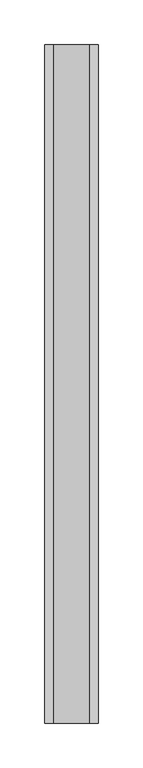
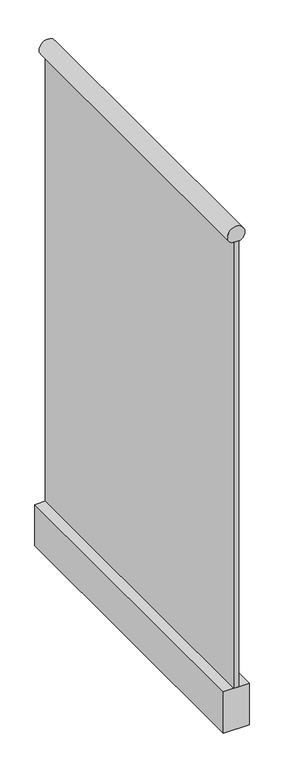
"""IFC4 building model written with IfcOpenShell, lengths in millimetres: railing geometry."""

from ifc_helpers import new_model, si_unit, point, frame, frame_2d, origin, place, context, project, spatial, polyline, circle_curve, trimmed, segment, composite_curve, outline, extrude, source, transform, mapped, element, save


def railing_f1bd4664(model_context):
    return source(origin(), model_context, "Body", "SweptSolid", [
        extrude(outline(composite_curve([segment(trimmed(circle_curve(frame_2d((5015.3205081, -1533.8712297)), 20.0), [point((4998.0, -1523.8712297))], [point((4998.0, -1543.8712297))], False, "CARTESIAN"), True, "CONTINUOUS"), segment(polyline([(4998.0, -1543.8712297), (4998.0, -1523.8712297)]), True, "CONTINUOUS")], self_intersect=False)), frame((0.0, -6422.0014262, 0.0), z_axis=(0.0, 1.0, 0.0), x_axis=(0.0, 0.0, 1.0)), (0.0, 0.0, 1.0), 760.0),
        extrude(outline(polyline([(-1527.8712297, -6422.0014262), (-1539.8712297, -6422.0014262), (-1539.8712297, -5662.0014262), (-1527.8712297, -5662.0014262), (-1527.8712297, -6422.0014262)])), frame((0.0, 0.0, 3900.0), z_axis=(0.0, 0.0, 1.0), x_axis=(1.0, 0.0, 0.0)), (0.0, 0.0, 1.0), 1098.0),
        extrude(outline(polyline([(-1503.8712297, -6422.0014262), (-1563.8712297, -6422.0014262), (-1563.8712297, -5662.0014262), (-1503.8712297, -5662.0014262), (-1503.8712297, -6422.0014262)])), frame((0.0, 0.0, 3798.0), z_axis=(0.0, 0.0, 1.0), x_axis=(1.0, 0.0, 0.0)), (0.0, 0.0, 1.0), 102.0),
    ])


if __name__ == "__main__":
    model = new_model("IFC4")
    model_context = context("Model", 3, world=origin())
    ifc_project = project(units=[si_unit("LENGTHUNIT", "METRE", prefix="MILLI")], contexts=[model_context])
    site = spatial("IfcSite", under=ifc_project)
    building = spatial("IfcBuilding", under=site)
    placement = place(None, origin())
    railing_shape = railing_f1bd4664(model_context)
    element("IfcRailing", 1, at=placement, inside=building, context=model_context, shape_type="MappedRepresentation", body=[
        mapped(railing_shape, transform((0.0, 0.0, 0.0), x_axis=(1.0, 0.0, 0.0), y_axis=(0.0, 1.0, 0.0), z_axis=(0.0, 0.0, 1.0))),
    ])
    save(model, "model.ifc")

# Revit data of these elements
# Element 1 (IfcRailing)
#   Materials on its faces: "Metal - Aluminum"
# Materials
#   "Metal - Aluminum": colour RGB 247 247 247, transparency 0, Cost = 0
